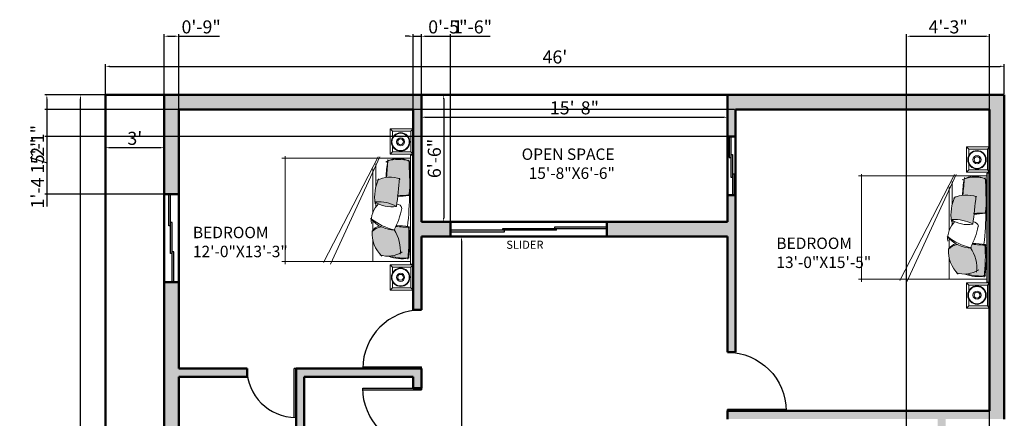
# Model space of a CAD drawing. Units: inches. Extents: x 1913 to 5309, y 1003 to 1733.
# Tile 12 of 23: x 2595 to 3199, y 1488 to 1733. Entities that reach past the tile are written whole.
import ezdxf

# ---------------------------------------------------------------- set-up
doc = ezdxf.new("R2010")
doc.units = ezdxf.units.IN
for name, color, linetype, lineweight in [('0.10', 252, 'Continuous', 9), ('0.15', 34, 'Continuous', 15), ('A-ANNO-DIMS', 2, 'Continuous', 18), ('A-ANNO-TEXT', 7, 'Continuous', 18), ('A-AREA-IDEN', 3, 'Continuous', 18), ('A-DOOR', 4, 'Continuous', 25), ('A-FLOR-PATT', 252, 'Continuous', 13), ('A-FURN', 8, 'Continuous', 18), ('A-FURN-PATT', 8, 'Continuous', 13), ('A-GLAZ', 5, 'Continuous', 25), ('A-WALL', 7, 'Continuous', 50)]:
    doc.layers.add(name, color=color, linetype=linetype, lineweight=lineweight)
doc.styles.get("Standard").update_dxf_attribs({"font": 'arial.ttf'})
doc.dimstyles.new('ISO-25', dxfattribs={"dimtxt": 8, "dimasz": 2.5, "dimexe": 1.25, "dimexo": 0.625, "dimtad": 1, "dimdec": 1, "dimlunit": 3, "dimtxsty": 'Standard', "dimcen": 2.5, "dimclrd": 256, "dimclrt": 1, "dimadec": 0, "dimazin": 0, "dimtfac": 1, "dimtdec": 1, "dimtmove": 0, "dimatfit": 3, "dimfxl": 1, "dimarcsym": 0})

# ---------------------------------------------------------------- blocks, each defined once
blk = doc.blocks.new('camita')
at = {"layer": '0.10'}
for p, q in [((-0.85, -0.045), (0.85, -0.045)), ((-0.805, -0.045), (-0.805, -2.048)), ((0.805, -0.045), (0.805, -2.048)), ((-0.827, -0.521), (0.846, -1.293)), ((-0.827, -0.548), (0.824, -1.399)), ((-0.716, -0.585), (-0.355, -0.585)), ((-0.114, -0.585), (-0.049, -0.585)), ((-0.638, -0.63), (0.043, -0.63)), ((0.175, -0.63), (0.318, -0.63)), ((0.474, -0.63), (0.805, -0.63)), ((-0.835, -2), (0.846, -2))]:
    blk.add_line(p, q, dxfattribs=at)
blk.add_lwpolyline([(-0.85, -0.041), (0.85, -0.041), (0.85, 0), (-0.85, 0)], close=True, dxfattribs=at)
for centre, radius, start, end in [((-0.457, -0.236), 0.344, 147.51, 213.8336), ((-0.2, -0.227), 0.586, 163.9263, 197.1409), ((-0.364, -5.846), 5.791, 83.8073, 94.1211), ((-0.51, -1.723), 1.678, 80.1255, 98.6619), ((2.353, -0.053), 2.58, 180.1063, 184.3854), ((-1.544, -0.245), 1.333, 359.9394, 7.5533), ((1.581, -0.289), 1.335, 170.3802, 178.9914), ((-1.44, -0.061), 1.712, 352.9291, 0.3959), ((0.452, -3.067), 3, 83.9026, 93.6759), ((0.486, -1.629), 1.578, 80.1602, 98.06), ((0.029, -0.138), 0.726, 342.5841, 6.0048), ((0.133, -0.17), 0.631, 339.923, 8.7433), ((-0.054, -0.363), 0.454, 159.3026, 206.5026), ((-1.33, -9.675), 9.499, 82.2708, 84.9399), ((0.458, -0.545), 0.584, 151.0456, 184.1497), ((-0.534, -0.339), 0.487, 327.2644, 9.0473), ((-0.007, -0.258), 0.0828, 100.018, 179.736), ((-0.293, -1.438), 1.29, 61.9749, 77.8435), ((-0.199, -0.274), 0.516, 310.7395, 359.0576), ((-0.567, -0.087), 0.906, 321.6953, 346.4626), ((0.627, -0.752), 0.551, 82.9691, 124.6739), ((0.32, -0.394), 0.404, 341.4524, 33.4512), ((-1.867, -14.986), 14.632, 84.6597, 85.7516), ((-0.46, 1.486), 1.909, 260.953, 268.6517), ((-0.2, 0.064), 0.667, 244.7809, 279.0606), ((0.179, -0.272), 0.383, 224.5284, 275.2229), ((0.438, -0.483), 0.19, 193.6849, 236.7035), ((0.571, -0.432), 0.315, 192.9388, 221.9636), ((0.361, -0.133), 0.51, 267.2589, 315.2997)]:
    blk.add_arc(centre, radius, start, end, dxfattribs=at)
blk = doc.blocks.new('VELADOR')
at = {"layer": '0.15'}
for p, q in [((-0.248, 0), (-0.203, -0.045)), ((0.248, 0), (0.202, -0.045)), ((-0.203, -0.405), (-0.248, -0.45)), ((0.248, -0.45), (0.202, -0.405))]:
    blk.add_line(p, q, dxfattribs=at)
blk.add_lwpolyline([(-0.248, 0), (-0.248, -0.45), (0.248, -0.45), (0.248, 0)], close=True, dxfattribs=at)
blk.add_lwpolyline([(0.092, -0.405), (0.202, -0.405), (0.202, -0.045), (-0.203, -0.045), (-0.203, -0.405), (-0.082, -0.405)], dxfattribs=at)
for radius in [0.18, 0.169, 0.0788, 0.0563]:
    blk.add_circle((0.005, -0.247), radius, dxfattribs=at)
blk = doc.blocks.new('*D41')
at = {"layer": 'A-ANNO-DIMS', "color": 0, "lineweight": -2, "transparency": 16777216}
for p, q in [((2646.71, 1686.96), (2630.73, 1686.96)), ((2631.98, 1101.46), (2631.98, 1684.46)), ((2646.71, 1098.96), (2630.73, 1098.96))]:
    blk.add_line(p, q, dxfattribs=at)
at = {"layer": 'A-ANNO-DIMS', "color": 0, "transparency": 16777216}
for points in [[(2631.56, 1684.46), (2632.4, 1684.46), (2631.98, 1686.96)], [(2631.56, 1101.46), (2632.4, 1101.46), (2631.98, 1098.96)]]:
    blk.add_solid(points, dxfattribs=at)
at = {"layer": 'Defpoints', "color": 0, "transparency": 16777216}
for p in [(2631.98, 1686.96), (2647.34, 1686.96), (2647.34, 1098.96)]:
    blk.add_point(p, dxfattribs=at)
at = {"layer": 'A-ANNO-DIMS', "color": 0, "transparency": 16777216, "insert": (2627.27, 1392.96), "char_height": 8, "attachment_point": 5, "rotation": 90}
blk.add_mtext("49'", dxfattribs=at)
blk = doc.blocks.new('*D42')
at = {"layer": 'A-ANNO-DIMS', "color": 0, "lineweight": -2, "transparency": 16777216}
for p, q in [((2647.34, 1687.59), (2647.34, 1705.75)), ((3199.34, 1687.59), (3199.34, 1705.75)), ((2649.84, 1704.5), (3196.84, 1704.5))]:
    blk.add_line(p, q, dxfattribs=at)
at = {"layer": 'A-ANNO-DIMS', "color": 0, "transparency": 16777216}
for points in [[(2649.84, 1704.92), (2649.84, 1704.08), (2647.34, 1704.5)], [(3196.84, 1704.92), (3196.84, 1704.08), (3199.34, 1704.5)]]:
    blk.add_solid(points, dxfattribs=at)
at = {"layer": 'Defpoints', "color": 0, "transparency": 16777216}
for p in [(3199.34, 1704.5), (2647.34, 1686.96), (3199.34, 1686.96)]:
    blk.add_point(p, dxfattribs=at)
at = {"layer": 'A-ANNO-DIMS', "color": 0, "transparency": 16777216, "insert": (2923.34, 1709.21), "char_height": 8, "attachment_point": 5}
blk.add_mtext("46'", dxfattribs=at)
blk = doc.blocks.new('*D43')
at = {"layer": 'A-ANNO-DIMS', "color": 0, "lineweight": -2, "transparency": 16777216}
for p, q in [((2841.34, 1679.78), (2841.34, 1672.02)), ((3029.34, 1679.78), (3029.34, 1672.02)), ((2843.84, 1673.27), (3026.84, 1673.27))]:
    blk.add_line(p, q, dxfattribs=at)
at = {"layer": 'A-ANNO-DIMS', "color": 0, "transparency": 16777216}
for points in [[(2843.84, 1673.68), (2843.84, 1672.85), (2841.34, 1673.27)], [(3026.84, 1673.68), (3026.84, 1672.85), (3029.34, 1673.27)]]:
    blk.add_solid(points, dxfattribs=at)
at = {"layer": 'Defpoints', "color": 0, "transparency": 16777216}
for p in [(2841.34, 1680.41), (3029.34, 1680.41), (3029.34, 1673.27)]:
    blk.add_point(p, dxfattribs=at)
at = {"layer": 'A-ANNO-DIMS', "color": 0, "transparency": 16777216, "insert": (2935.34, 1677.98), "char_height": 8, "attachment_point": 5}
blk.add_mtext('15\'-8"', dxfattribs=at)
blk = doc.blocks.new('*D44')
at = {"layer": 'A-ANNO-DIMS', "color": 0, "lineweight": -2, "transparency": 16777216}
for p, q in [((2855.15, 1686.96), (2853.78, 1686.96)), ((2855.03, 1684.46), (2855.03, 1611.46)), ((2855.15, 1608.96), (2853.78, 1608.96))]:
    blk.add_line(p, q, dxfattribs=at)
at = {"layer": 'A-ANNO-DIMS', "color": 0, "transparency": 16777216}
for points in [[(2854.61, 1684.46), (2855.44, 1684.46), (2855.03, 1686.96)], [(2854.61, 1611.46), (2855.44, 1611.46), (2855.03, 1608.96)]]:
    blk.add_solid(points, dxfattribs=at)
at = {"layer": 'Defpoints', "color": 0, "transparency": 16777216}
for p in [(2855.78, 1686.96), (2855.03, 1608.96), (2855.78, 1608.96)]:
    blk.add_point(p, dxfattribs=at)
at = {"layer": 'A-ANNO-DIMS', "color": 0, "transparency": 16777216, "insert": (2850.32, 1647.96), "char_height": 8, "attachment_point": 5, "rotation": 90}
blk.add_mtext('6\'-6"', dxfattribs=at)
blk = doc.blocks.new('*D45')
at = {"layer": 'A-ANNO-DIMS', "color": 0, "lineweight": -2, "transparency": 16777216}
for p, q in [((2647.34, 1655.19), (2647.34, 1655.82)), ((2680.84, 1654.57), (2649.84, 1654.57)), ((2683.34, 1655.19), (2683.34, 1655.82))]:
    blk.add_line(p, q, dxfattribs=at)
at = {"layer": 'A-ANNO-DIMS', "color": 0, "transparency": 16777216}
for points in [[(2649.84, 1654.99), (2649.84, 1654.15), (2647.34, 1654.57)], [(2680.84, 1654.99), (2680.84, 1654.15), (2683.34, 1654.57)]]:
    blk.add_solid(points, dxfattribs=at)
at = {"layer": 'Defpoints', "color": 0, "transparency": 16777216}
for p in [(2647.34, 1654.57), (2647.34, 1654.57), (2683.34, 1654.57)]:
    blk.add_point(p, dxfattribs=at)
at = {"layer": 'A-ANNO-DIMS', "color": 0, "transparency": 16777216, "insert": (2665.34, 1659.28), "char_height": 8, "attachment_point": 5}
blk.add_mtext("3'", dxfattribs=at)
blk = doc.blocks.new('*D48')
at = {"layer": 'A-ANNO-DIMS', "color": 0, "lineweight": -2, "transparency": 16777216}
for p, q in [((2859.93, 1599.96), (2867.23, 1599.96)), ((2865.98, 1597.46), (2865.98, 1158.43)), ((2859.93, 1155.93), (2867.23, 1155.93))]:
    blk.add_line(p, q, dxfattribs=at)
at = {"layer": 'A-ANNO-DIMS', "color": 0, "transparency": 16777216}
for points in [[(2865.56, 1597.46), (2866.39, 1597.46), (2865.98, 1599.96)], [(2865.56, 1158.43), (2866.39, 1158.43), (2865.98, 1155.93)]]:
    blk.add_solid(points, dxfattribs=at)
at = {"layer": 'Defpoints', "color": 0, "transparency": 16777216}
for p in [(2859.31, 1599.96), (2859.31, 1155.93), (2865.98, 1155.93)]:
    blk.add_point(p, dxfattribs=at)
at = {"layer": 'A-ANNO-DIMS', "color": 0, "transparency": 16777216, "insert": (2861.26, 1377.95), "char_height": 8, "attachment_point": 5, "rotation": 90}
blk.add_mtext("37'", dxfattribs=at)
blk = doc.blocks.new("D1 3'")
for p, q in [((0, 36), (0, 0)), ((1, 36), (1, 0)), ((0, 0), (1, 0))]:
    blk.add_line(p, q)
blk.add_arc((0, 0), 36, 0, 90)
blk = doc.blocks.new("D2 2'6")
for p, q in [((0, 30), (0, 0)), ((1, 30), (1, 0)), ((0, 0), (1, 0))]:
    blk.add_line(p, q)
blk.add_arc((0, 0), 30, 0, 90)
blk = doc.blocks.new('WIN-54')
for p, q in [((0, 54), (0, 35)), ((1, 54), (1, 17)), ((0, 35), (1, 35)), ((1, 36), (2, 36)), ((2, 36), (2, 0)), ((2, 19), (3, 19)), ((3, 19), (3, 0)), ((1, 17), (2, 17))]:
    blk.add_line(p, q)
blk = doc.blocks.new('WIN-36')
for p, q in [((0, 23), (0, 36)), ((1, 11), (1, 36)), ((2, 25), (1, 25)), ((2, 0), (2, 25)), ((1, 23), (0, 23)), ((3, 13), (2, 13)), ((3, 0), (3, 13)), ((2, 11), (1, 11))]:
    blk.add_line(p, q)
blk = doc.blocks.new('WIN-SLIDER-96')
for p, q in [((65, 1), (0, 1)), ((0, 0), (33, 0)), ((32, 2), (96, 2)), ((32, 1), (32, 2)), ((33, 0), (33, 1)), ((64, 3), (96, 3)), ((64, 2), (64, 3)), ((65, 1), (65, 2))]:
    blk.add_line(p, q)
blk = doc.blocks.new('*D116')
at = {"layer": 'A-ANNO-DIMS', "color": 0, "lineweight": -2, "transparency": 16777216}
for p, q in [((2683.34, 1687.59), (2683.34, 1724.21)), ((2692.34, 1678.59), (2692.34, 1724.21))]:
    blk.add_line(p, q, dxfattribs=at)
at = {"layer": 'A-ANNO-DIMS', "lineweight": -2, "transparency": 16777216}
for p, q in [((2685.84, 1722.96), (2689.84, 1722.96)), ((2692.34, 1722.96), (2717.35, 1722.96))]:
    blk.add_line(p, q, dxfattribs=at)
at = {"layer": 'A-ANNO-DIMS', "transparency": 16777216}
for points in [[(2685.84, 1723.38), (2685.84, 1722.55), (2683.34, 1722.96)], [(2689.84, 1723.38), (2689.84, 1722.55), (2692.34, 1722.96)]]:
    blk.add_solid(points, dxfattribs=at)
at = {"layer": 'Defpoints', "color": 0, "transparency": 16777216}
for p in [(2692.34, 1722.96), (2683.34, 1686.96), (2692.34, 1677.96)]:
    blk.add_point(p, dxfattribs=at)
at = {"layer": 'A-ANNO-DIMS', "color": 1, "transparency": 16777216, "insert": (2706.1, 1727.67), "char_height": 8, "attachment_point": 5}
blk.add_mtext('0\'-9"', dxfattribs=at)
blk = doc.blocks.new('*D117')
at = {"layer": 'A-ANNO-DIMS', "color": 0, "lineweight": -2, "transparency": 16777216}
for p, q in [((2836.34, 1678.59), (2836.34, 1724.21)), ((2841.34, 1687.59), (2841.34, 1724.21))]:
    blk.add_line(p, q, dxfattribs=at)
at = {"layer": 'A-ANNO-DIMS', "lineweight": -2, "transparency": 16777216}
for p, q in [((2833.84, 1722.96), (2831.34, 1722.96)), ((2836.34, 1722.96), (2841.34, 1722.96)), ((2843.84, 1722.96), (2868.85, 1722.96))]:
    blk.add_line(p, q, dxfattribs=at)
at = {"layer": 'A-ANNO-DIMS', "transparency": 16777216}
for points in [[(2833.84, 1723.38), (2833.84, 1722.55), (2836.34, 1722.96)], [(2843.84, 1723.38), (2843.84, 1722.55), (2841.34, 1722.96)]]:
    blk.add_solid(points, dxfattribs=at)
at = {"layer": 'Defpoints', "color": 0, "transparency": 16777216}
for p in [(2841.34, 1722.96), (2841.34, 1686.96), (2836.34, 1677.96)]:
    blk.add_point(p, dxfattribs=at)
at = {"layer": 'A-ANNO-DIMS', "color": 1, "transparency": 16777216, "insert": (2857.6, 1727.67), "char_height": 8, "attachment_point": 5}
blk.add_mtext('0\'-5"', dxfattribs=at)
blk = doc.blocks.new('*D118')
at = {"layer": 'A-ANNO-DIMS', "color": 0, "lineweight": -2, "transparency": 16777216}
for p, q in [((2682.71, 1686.96), (2610.09, 1686.96)), ((2682.71, 1625.96), (2610.09, 1625.96))]:
    blk.add_line(p, q, dxfattribs=at)
at = {"layer": 'A-ANNO-DIMS', "lineweight": -2, "transparency": 16777216}
blk.add_line((2611.34, 1684.46), (2611.34, 1628.46), dxfattribs=at)
at = {"layer": 'A-ANNO-DIMS', "transparency": 16777216}
for points in [[(2610.92, 1684.46), (2611.76, 1684.46), (2611.34, 1686.96)], [(2610.92, 1628.46), (2611.76, 1628.46), (2611.34, 1625.96)]]:
    blk.add_solid(points, dxfattribs=at)
at = {"layer": 'Defpoints', "color": 0, "transparency": 16777216}
for p in [(2683.34, 1686.96), (2611.34, 1625.96), (2683.34, 1625.96)]:
    blk.add_point(p, dxfattribs=at)
at = {"layer": 'A-ANNO-DIMS', "color": 1, "transparency": 16777216, "insert": (2606.63, 1656.46), "char_height": 8, "attachment_point": 5, "rotation": 90}
blk.add_mtext('5\'-1"', dxfattribs=at)
blk = doc.blocks.new('*D120')
at = {"layer": 'A-ANNO-DIMS', "color": 0, "lineweight": -2, "transparency": 16777216}
for p, q in [((3033.71, 1677.96), (2610.09, 1677.96)), ((3033.71, 1661.46), (2610.09, 1661.46))]:
    blk.add_line(p, q, dxfattribs=at)
at = {"layer": 'A-ANNO-DIMS', "lineweight": -2, "transparency": 16777216}
for p, q in [((2611.34, 1675.46), (2611.34, 1663.96)), ((2611.34, 1661.46), (2611.34, 1618.56))]:
    blk.add_line(p, q, dxfattribs=at)
at = {"layer": 'A-ANNO-DIMS', "transparency": 16777216}
for points in [[(2610.92, 1675.46), (2611.76, 1675.46), (2611.34, 1677.96)], [(2610.92, 1663.96), (2611.76, 1663.96), (2611.34, 1661.46)]]:
    blk.add_solid(points, dxfattribs=at)
at = {"layer": 'Defpoints', "color": 0, "transparency": 16777216}
for p in [(3034.34, 1677.96), (2611.34, 1661.46), (3034.34, 1661.46)]:
    blk.add_point(p, dxfattribs=at)
at = {"layer": 'A-ANNO-DIMS', "color": 1, "transparency": 16777216, "insert": (2606.58, 1638.76), "char_height": 8, "attachment_point": 5, "rotation": 90}
blk.add_mtext('1\'-4 1/2"', dxfattribs=at)
blk = doc.blocks.new('*D121')
at = {"layer": 'A-ANNO-DIMS', "color": 0, "lineweight": -2, "transparency": 16777216}
for p, q in [((2841.34, 1609.59), (2841.34, 1724.21)), ((2859.31, 1609.59), (2859.31, 1724.21))]:
    blk.add_line(p, q, dxfattribs=at)
at = {"layer": 'A-ANNO-DIMS', "lineweight": -2, "transparency": 16777216}
for p, q in [((2843.84, 1722.96), (2856.81, 1722.96)), ((2859.31, 1722.96), (2883.57, 1722.96))]:
    blk.add_line(p, q, dxfattribs=at)
at = {"layer": 'A-ANNO-DIMS', "transparency": 16777216}
for points in [[(2843.84, 1723.38), (2843.84, 1722.55), (2841.34, 1722.96)], [(2856.81, 1723.38), (2856.81, 1722.55), (2859.31, 1722.96)]]:
    blk.add_solid(points, dxfattribs=at)
at = {"layer": 'Defpoints', "color": 0, "transparency": 16777216}
for p in [(2859.31, 1722.96), (2841.34, 1608.96), (2859.31, 1608.96)]:
    blk.add_point(p, dxfattribs=at)
at = {"layer": 'A-ANNO-DIMS', "color": 1, "transparency": 16777216, "insert": (2872.69, 1727.67), "char_height": 8, "attachment_point": 5}
blk.add_mtext('1\'-6"', dxfattribs=at)
blk = doc.blocks.new('*D126')
at = {"layer": 'A-ANNO-DIMS', "color": 0, "lineweight": -2, "transparency": 16777216}
for p, q in [((3139.34, 1180.59), (3139.34, 1724.21)), ((3190.34, 1180.59), (3190.34, 1724.21))]:
    blk.add_line(p, q, dxfattribs=at)
at = {"layer": 'A-ANNO-DIMS', "lineweight": -2, "transparency": 16777216}
blk.add_line((3141.84, 1722.96), (3187.84, 1722.96), dxfattribs=at)
at = {"layer": 'A-ANNO-DIMS', "transparency": 16777216}
for points in [[(3141.84, 1723.38), (3141.84, 1722.55), (3139.34, 1722.96)], [(3187.84, 1723.38), (3187.84, 1722.55), (3190.34, 1722.96)]]:
    blk.add_solid(points, dxfattribs=at)
at = {"layer": 'Defpoints', "color": 0, "transparency": 16777216}
for p in [(3190.34, 1722.96), (3139.34, 1179.96), (3190.34, 1179.96)]:
    blk.add_point(p, dxfattribs=at)
at = {"layer": 'A-ANNO-DIMS', "color": 1, "transparency": 16777216, "insert": (3164.84, 1727.68), "char_height": 8, "attachment_point": 5}
blk.add_mtext('4\'-3"', dxfattribs=at)

msp = doc.modelspace()

# ---------------------------------------------------------------- hatches: boundary and pattern name
at = {"layer": 'A-FLOR-PATT'}
h = msp.add_hatch(color=256, dxfattribs=at)
h.dxf.hatch_style = 1
h.paths.add_polyline_path([(2841.34, 1686.96), (2683.34, 1686.96), (2683.34, 1625.96), (2692.34, 1625.96), (2692.34, 1677.96), (2836.34, 1677.96), (2836.34, 1554.96), (2841.34, 1554.96), (2841.34, 1599.96), (2859.31, 1599.96), (2859.31, 1608.96), (2841.34, 1608.96)])
h.paths.add_polyline_path([(3034.34, 1625.46), (3029.34, 1625.46), (3029.34, 1608.96), (2955.31, 1608.96), (2955.31, 1599.96), (3029.34, 1599.96), (3029.34, 1528.96), (3034.34, 1528.96)])
h.paths.add_polyline_path([(3199.34, 1686.96), (3029.34, 1686.96), (3029.34, 1661.46), (3034.34, 1661.46), (3034.34, 1677.96), (3190.34, 1677.96), (3190.34, 1492.96), (3029.34, 1492.96), (3029.34, 1487.96), (3158.34, 1487.96), (3158.34, 1464.96), (3163.34, 1464.96), (3163.34, 1487.96), (3199.34, 1487.96)])
h.paths.add_polyline_path([(3099.34, 1400.96), (3163.34, 1400.96), (3163.34, 1428.96), (3158.34, 1428.96), (3158.34, 1405.96), (3029.34, 1405.96), (3029.34, 1311.96), (3034.34, 1311.96), (3034.34, 1323.96), (3058.34, 1323.96), (3058.34, 1328.96), (3034.34, 1328.96), (3034.34, 1400.96), (3094.34, 1400.96), (3094.34, 1358.96), (3099.34, 1358.96)])
h.paths.add_polyline_path([(3199.34, 1405.96), (3187.34, 1405.96), (3187.34, 1400.96), (3190.34, 1400.96), (3190.34, 1328.96), (3094.34, 1328.96), (3094.34, 1323.96), (3190.34, 1323.96), (3190.34, 1299.96), (3190.34, 1179.96), (3176.2, 1179.96), (3139.34, 1179.96), (3139.34, 1170.96), (3190.34, 1170.96), (3190.34, 1146.96), (3199.34, 1146.96)])
h.paths.add_polyline_path([(3085.34, 1179.96), (3064.34, 1179.96), (3064.34, 1170.96), (3085.34, 1170.96)])
h.paths.add_polyline_path([(3029.34, 1158.98), (3029.34, 1199.59, 0.414216), (3026.32, 1202.59), (3010.47, 1202.59, 0.414214), (3007.47, 1199.59), (3007.47, 1181.52, 0.46174), (3009.2, 1180.04), (3026.11, 1180.04, 0.414263), (3025.52, 1179.45), (3025.52, 1162.57, 0.41435), (3026.11, 1161.97), (3007.38, 1161.97, 0.41842), (3006.78, 1161.36, 0.785879), (3005.87, 1162.09, 0.298637), (3006.77, 1163.46), (3006.77, 1178.53, 0.414214), (3005.27, 1180.02), (2990.22, 1180.02, 0.416116), (2988.72, 1178.51, 0.414208), (2987.21, 1180.02), (2987.2, 1180.02, -0.413869), (2988.7, 1178.52, -0.412492), (2990.21, 1180.02), (2990.21, 1180.03), (3005.27, 1180.02, -0.414213), (3006.77, 1178.53, -0.414214), (3008.27, 1180.02), (3008.14, 1180.27, -0.252555), (3007.47, 1181.52), (3007.45, 1181.51), (3007.47, 1199.59, -0.414214), (3010.47, 1202.59), (3026.33, 1202.59, -0.414214), (3029.34, 1199.59), (3029.34, 1275.96), (3034.34, 1275.96), (3034.34, 1146.96), (3011.34, 1146.96), (3011.34, 1155.96), (2951.06, 1155.96, -0.414214), (2948.06, 1158.97), (2948.06, 1158.97, 0.421637), (2951.14, 1155.96), (3026.4, 1155.96, 0.407251)])
h.paths.add_polyline_path([(2845.34, 1275.96), (2836.34, 1275.96), (2836.34, 1233.96), (2845.34, 1233.96), (2845.34, 1237.71)])
h.paths.add_polyline_path([(2845.34, 1173.96), (2836.34, 1173.96), (2836.34, 1146.96), (2863.34, 1146.96), (2863.34, 1155.93), (2848.48, 1155.93, -0.414214), (2845.34, 1159.07)])
h.paths.add_polyline_path([(2841.34, 1356.96), (2836.34, 1356.96), (2836.34, 1328.96), (2793.34, 1328.96), (2793.34, 1405.96), (2841.34, 1405.96), (2841.34, 1470.96), (2836.34, 1470.96), (2836.34, 1410.96), (2769.34, 1410.96), (2769.34, 1513.96), (2836.34, 1513.96), (2836.34, 1506.96), (2841.34, 1506.96), (2841.34, 1518.96), (2764.34, 1518.96), (2764.34, 1405.96), (2788.34, 1405.96), (2788.34, 1328.96), (2692.34, 1328.96), (2692.34, 1340.96), (2683.34, 1340.96), (2683.34, 1323.96), (2841.34, 1323.96)])
h.paths.add_polyline_path([(2692.34, 1513.96), (2734.34, 1513.96), (2734.34, 1518.96), (2692.34, 1518.96), (2692.34, 1571.96), (2683.34, 1571.96), (2683.34, 1420.96), (2683.34, 1364.96), (2692.34, 1364.96), (2692.34, 1405.96), (2734.34, 1405.96), (2734.34, 1410.96), (2692.34, 1410.96)])
at = {"layer": 'A-FURN-PATT'}
h = msp.add_hatch(color=256, dxfattribs=at)
h.dxf.hatch_style = 1
h.paths.add_polyline_path([(2819.91, 1636.36, -0.113891), (2827.91, 1635.49, -0.006967), (2826.83, 1625.13, -0.016701), (2833.61, 1625.4, 0.015442), (2834.18, 1629.44, 0.01851), (2833.65, 1646.31, 0.020657), (2832.66, 1646.81, 0.131047), (2820.76, 1646.43, -0.004387)])
h.paths.add_polyline_path([(2825.64, 1606.26, -0.011742), (2824.57, 1604.13, -0.175864), (2828.33, 1589.82, -0.098488), (2822.39, 1588.01, 0.094792), (2833.07, 1586.79, 0.040212), (2833.45, 1605.75, -0.029051)])
h = msp.add_hatch(color=256, dxfattribs=at)
h.dxf.hatch_style = 1
h.paths.add_polyline_path([(2812.77, 1621.24, 0.181694), (2826, 1618.54, 0.011408), (2827.91, 1635.49, 0.189536), (2814.83, 1634.97, 0.134508)])
h.paths.add_polyline_path([(2824.67, 1603.99, -0.104045), (2816.57, 1606.06, 0.127326), (2811.06, 1603.2, 0.202559), (2816.44, 1588.54, 0.194952), (2828.33, 1589.82, 0.173835)])
h = msp.add_hatch(color=256, dxfattribs=at)
h.dxf.hatch_style = 1
h.paths.add_polyline_path([(3173.91, 1625.42, -0.113891), (3181.91, 1624.55, -0.006967), (3180.83, 1614.18, -0.016701), (3187.61, 1614.45, 0.015442), (3188.18, 1618.49, 0.01851), (3187.65, 1635.36, 0.020657), (3186.66, 1635.87, 0.131047), (3174.76, 1635.49, -0.004387)])
h.paths.add_polyline_path([(3179.64, 1595.32, -0.011742), (3178.57, 1593.19, -0.175864), (3182.33, 1578.88, -0.098488), (3176.39, 1577.06, 0.094792), (3187.07, 1575.85, 0.040212), (3187.45, 1594.81, -0.029051)])
h = msp.add_hatch(color=256, dxfattribs=at)
h.dxf.hatch_style = 1
h.paths.add_polyline_path([(3166.76, 1610.37, -0.150361), (3180, 1607.59, 0.011408), (3181.91, 1624.55, 0.189536), (3168.83, 1624.03, 0.133776)])
h.paths.add_polyline_path([(3178.67, 1593.05, -0.104045), (3170.57, 1595.12, 0.127326), (3165.06, 1592.26, 0.202559), (3170.44, 1577.6, 0.194952), (3182.33, 1578.88, 0.173835)])

# ---------------------------------------------------------------- linework, layer by layer
at = {"layer": 'A-WALL'}
for p, q in [((2647.34, 1686.96), (3199.34, 1686.96)), ((2647.34, 1098.96), (2647.34, 1686.96)), ((2683.34, 1686.96), (2683.34, 1420.96)), ((2841.34, 1686.96), (2841.34, 1608.96)), ((3029.34, 1686.96), (3029.34, 1608.96)), ((3199.34, 1686.96), (3199.34, 1487.96)), ((2692.34, 1677.96), (2836.34, 1677.96)), ((2692.34, 1677.96), (2692.34, 1518.96)), ((2836.34, 1677.96), (2836.34, 1554.96)), ((3034.34, 1677.96), (3190.34, 1677.96)), ((3034.34, 1677.96), (3034.34, 1528.96)), ((3190.34, 1677.96), (3190.34, 1492.96)), ((3034.34, 1661.46), (3029.34, 1661.46)), ((2683.34, 1625.96), (2692.34, 1625.96)), ((3034.34, 1625.46), (3029.34, 1625.46)), ((2841.34, 1608.96), (3029.34, 1608.96)), ((2859.31, 1599.96), (2859.31, 1608.96)), ((2955.31, 1599.96), (2955.31, 1608.96)), ((2841.34, 1599.96), (3029.34, 1599.96)), ((2841.34, 1599.96), (2841.34, 1554.96)), ((3029.34, 1599.96), (3029.34, 1528.96)), ((2683.34, 1571.96), (2692.34, 1571.96)), ((2836.34, 1554.96), (2841.34, 1554.96)), ((3029.34, 1528.96), (3034.34, 1528.96)), ((2692.34, 1518.96), (2734.34, 1518.96)), ((2734.34, 1518.96), (2734.34, 1513.96)), ((2764.34, 1518.96), (2764.34, 1405.96)), ((2764.34, 1518.96), (2841.34, 1518.96)), ((2841.34, 1518.96), (2841.34, 1506.96)), ((2692.34, 1513.96), (2692.34, 1410.96)), ((2692.34, 1513.96), (2734.34, 1513.96)), ((2769.34, 1513.96), (2769.34, 1410.96)), ((2769.34, 1513.96), (2836.34, 1513.96)), ((2836.34, 1506.96), (2836.34, 1513.96)), ((2841.34, 1506.96), (2836.34, 1506.96)), ((3029.34, 1492.96), (3029.34, 1487.96)), ((3029.34, 1492.96), (3190.34, 1492.96))]:
    msp.add_line(p, q, dxfattribs=at)

# ---------------------------------------------------------------- block references
at = {"layer": 'A-DOOR'}
for name, p, rotation in [("D1 3'", (2841.34, 1518.96), 90), ("D2 2'6", (2764.21, 1518.96), 180)]:
    msp.add_blockref(name, p, dxfattribs=dict(at, rotation=rotation))
at = {"layer": 'A-DOOR', "xscale": -1}
for p, rotation in [((3029.34, 1492.96), 270), ((2841.34, 1506.96), 90)]:
    msp.add_blockref("D1 3'", p, dxfattribs=dict(at, rotation=rotation))
at = {"layer": 'A-FURN'}
for name, p, xscale, yscale, zscale, rotation in [('VELADOR', (2836.34, 1658.3), 31.41542173157097, 31.41542173157097, 31.41542173157097, 270), ('VELADOR', (3190.34, 1647.35), 31.41542173157097, 31.41542173157097, 31.41542173157097, 270), ('camita', (2836.34, 1616.46), 39.375, 39.375, 39.375, 270), ('camita', (3190.34, 1605.52), 39.375, 39.375, 39.375, 270), ('VELADOR', (2836.34, 1574.85), -31.41542173157097, 31.41542173157097, 31.41542173157097, 269.9999999999999), ('VELADOR', (3190.34, 1563.9), -31.41542173157097, 31.41542173157097, 31.41542173157097, 269.9999999999999)]:
    msp.add_blockref(name, p, dxfattribs=dict(at, xscale=xscale, yscale=yscale, zscale=zscale, rotation=rotation))
at = {"layer": 'A-GLAZ'}
for name, p, rotation in [('WIN-36', (3033.34, 1661.46), 180), ('WIN-54', (2689.32, 1625.59), 180.0440757868837)]:
    msp.add_blockref(name, p, dxfattribs=dict(at, rotation=rotation))
msp.add_blockref('WIN-SLIDER-96', (2859.31, 1602.96), dxfattribs=at)

# ---------------------------------------------------------------- texts
at = {"layer": 'A-ANNO-TEXT', "insert": (2893.51, 1597.49), "char_height": 5, "attachment_point": 1}
msp.add_mtext_dynamic_manual_height_columns('{SLIDER}', width=86.9528, gutter_width=12.5, heights=[5.17], dxfattribs=at)
at = {"layer": 'A-AREA-IDEN', "char_height": 7, "attachment_point": 1}
for s, width, insert in [('OPEN SPACE\\P  15\'-8"X6\'-6"', 115.9003, (2902.93, 1654.08)), ('BEDROOM\\P12\'-0"X13\'-3"', 86.9528, (2701.01, 1606.02)), ('BEDROOM\\P13\'-0"X15\'-5"', 86.9528, (3059.33, 1599.38))]:
    msp.add_mtext_dynamic_manual_height_columns(s, width=width, gutter_width=12.5, heights=[0], dxfattribs=dict(at, insert=insert))

# ---------------------------------------------------------------- dimensions: what is measured, and where the dimension line sits
at = {"layer": 'A-ANNO-DIMS'}
for base, p1, p2, override, picture, middle in [((2692.34, 1722.96), (2683.34, 1686.96), (2692.34, 1677.96), {"dimdec": 1, "dimlfac": 1, "dimrnd": 0, "dimzin": 1, "dimdsep": 46, "dimlunit": 4, "dimfrac": 2}, '*D116', (2706.1, 1727.67)), ((2841.34, 1722.96), (2836.34, 1677.96), (2841.34, 1686.96), {"dimdec": 1, "dimlfac": 1, "dimrnd": 0, "dimzin": 1, "dimdsep": 46, "dimlunit": 4, "dimfrac": 2}, '*D117', (2857.6, 1727.67)), ((2859.31, 1722.96), (2841.34, 1608.96), (2859.31, 1608.96), {"dimdec": 1, "dimlfac": 1, "dimrnd": 0, "dimzin": 1, "dimdsep": 46, "dimlunit": 4, "dimfrac": 2}, '*D121', (2872.69, 1727.67)), ((3190.34, 1722.96), (3139.34, 1179.96), (3190.34, 1179.96), {"dimdec": 1, "dimlfac": 1, "dimrnd": 0, "dimzin": 1, "dimdsep": 46, "dimlunit": 4, "dimfrac": 2}, '*D126', (3164.84, 1727.68)), ((3199.34, 1704.5), (2647.34, 1686.96), (3199.34, 1686.96), {"dimclrd": 0, "dimclre": 0, "dimclrt": 0}, '*D42', (2923.34, 1709.21)), ((3029.34, 1673.27), (2841.34, 1680.41), (3029.34, 1680.41), {"dimclrd": 0, "dimclre": 0, "dimclrt": 0}, '*D43', (2935.34, 1677.98)), ((2647.34, 1654.57), (2683.34, 1654.57), (2647.34, 1654.57), {"dimclrd": 0, "dimclre": 0, "dimclrt": 0}, '*D45', (2665.34, 1659.28))]:
    dim = msp.add_linear_dim(base=base, p1=p1, p2=p2, dimstyle='ISO-25', override=override, dxfattribs=at)
    dim.commit()
    dim.dimension.update_dxf_attribs({"geometry": picture, "text_midpoint": middle})
for base, p1, p2, override, picture, middle in [((2611.34, 1625.96), (2683.34, 1686.96), (2683.34, 1625.96), {"dimdec": 1, "dimlfac": 1, "dimrnd": 0, "dimzin": 1, "dimdsep": 46, "dimlunit": 4, "dimfrac": 2}, '*D118', (2606.63, 1656.46)), ((2631.98, 1686.96), (2647.34, 1098.96), (2647.34, 1686.96), {"dimclrd": 0, "dimclre": 0, "dimclrt": 0}, '*D41', (2627.27, 1392.96)), ((2855.03, 1608.96), (2855.78, 1686.96), (2855.78, 1608.96), {"dimclrd": 0, "dimclre": 0, "dimclrt": 0}, '*D44', (2850.32, 1647.96)), ((2611.34, 1661.46), (3034.34, 1677.96), (3034.34, 1661.46), {"dimdec": 1, "dimlfac": 1, "dimrnd": 0, "dimzin": 1, "dimdsep": 46, "dimlunit": 4, "dimfrac": 2}, '*D120', (2606.58, 1638.76)), ((2865.98, 1155.93), (2859.31, 1599.96), (2859.31, 1155.93), {"dimclrd": 0, "dimclre": 0, "dimclrt": 0}, '*D48', (2861.26, 1377.95))]:
    dim = msp.add_linear_dim(base=base, p1=p1, p2=p2, angle=90, dimstyle='ISO-25', override=override, dxfattribs=at)
    dim.commit()
    dim.dimension.update_dxf_attribs({"geometry": picture, "text_midpoint": middle})

doc.saveas('drawing.dxf')
